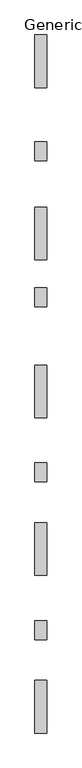
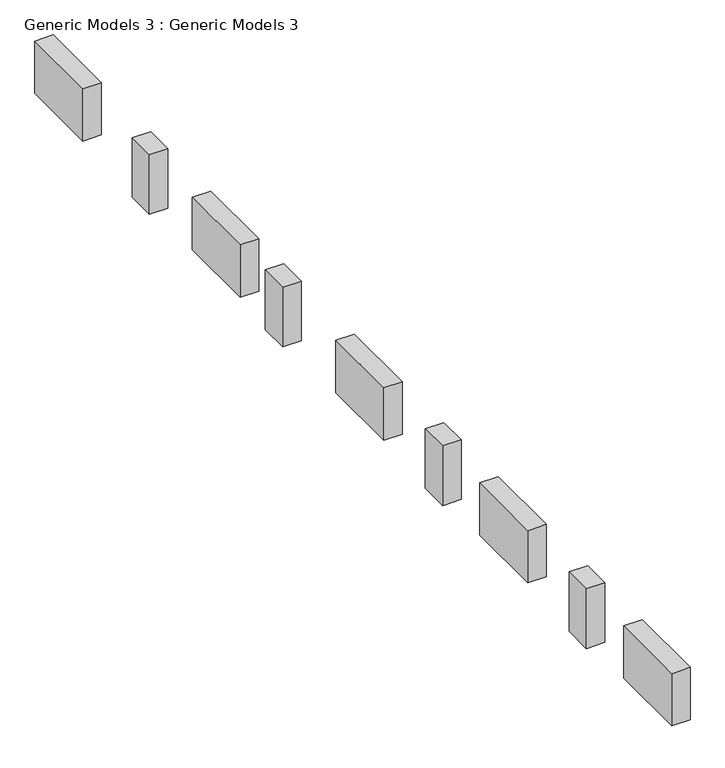
"""IFC4 building model written with IfcOpenShell, lengths in millimetres: proxy geometry, Generic Models 3 : Generic Models 3."""

from ifc_helpers import new_model, si_unit, frame, origin, place, context, project, spatial, polyline, outline, extrude, source, transform, mapped, element, save


def generic_models_3_generic_models_3_98a77e8e(model_context):
    return source(origin(), model_context, "Body", "SweptSolid", [
        extrude(outline(polyline([(5820.7206788, -7364.0778318), (5820.7206788, -8735.6778318), (5515.9206788, -8735.6778318), (5515.9206788, -7364.0778318), (5820.7206788, -7364.0778318)])), frame((0.0, 0.0, 262.9036405), z_axis=(0.0, 0.0, 1.0), x_axis=(1.0, 0.0, 0.0)), (0.0, 0.0, 1.0), 914.4),
        extrude(outline(polyline([(5820.7206788, -5805.4564015), (5820.7206788, -6300.7628124), (5515.9206788, -6300.7628124), (5515.9206788, -5805.4564015), (5820.7206788, -5805.4564015)])), frame((0.0, 0.0, 137.1997889), z_axis=(0.0, 0.0, 1.0), x_axis=(1.0, 0.0, 0.0)), (0.0, 0.0, 1.0), 1040.1038516),
        extrude(outline(polyline([(5820.7206788, -3249.2778318), (5820.7206788, -4620.8778318), (5515.9206788, -4620.8778318), (5515.9206788, -3249.2778318), (5820.7206788, -3249.2778318)])), frame((0.0, 0.0, 262.9036405), z_axis=(0.0, 0.0, 1.0), x_axis=(1.0, 0.0, 0.0)), (0.0, 0.0, 1.0), 914.4),
        extrude(outline(polyline([(5820.7206788, 862.0435985), (5820.7206788, -509.5564015), (5515.9206788, -509.5564015), (5515.9206788, 862.0435985), (5820.7206788, 862.0435985)])), frame((0.0, 0.0, 262.9036405), z_axis=(0.0, 0.0, 1.0), x_axis=(1.0, 0.0, 0.0)), (0.0, 0.0, 1.0), 914.4),
        extrude(outline(polyline([(5820.7206788, 4976.8435985), (5820.7206788, 3605.2435985), (5515.9206788, 3605.2435985), (5515.9206788, 4976.8435985), (5820.7206788, 4976.8435985)])), frame((0.0, 0.0, 262.9036405), z_axis=(0.0, 0.0, 1.0), x_axis=(1.0, 0.0, 0.0)), (0.0, 0.0, 1.0), 914.4),
        extrude(outline(polyline([(5820.7206788, 9472.6435985), (5820.7206788, 8101.0435985), (5515.9206788, 8101.0435985), (5515.9206788, 9472.6435985), (5820.7206788, 9472.6435985)])), frame((0.0, 0.0, 262.9036405), z_axis=(0.0, 0.0, 1.0), x_axis=(1.0, 0.0, 0.0)), (0.0, 0.0, 1.0), 914.4),
        extrude(outline(polyline([(5820.7206788, -1690.6564015), (5820.7206788, -2185.9628124), (5515.9206788, -2185.9628124), (5515.9206788, -1690.6564015), (5820.7206788, -1690.6564015)])), frame((0.0, 0.0, 137.1997889), z_axis=(0.0, 0.0, 1.0), x_axis=(1.0, 0.0, 0.0)), (0.0, 0.0, 1.0), 1040.1038516),
        extrude(outline(polyline([(5820.7206788, 2881.3435985), (5820.7206788, 2386.0371876), (5515.9206788, 2386.0371876), (5515.9206788, 2881.3435985), (5820.7206788, 2881.3435985)])), frame((0.0, 0.0, 137.1997889), z_axis=(0.0, 0.0, 1.0), x_axis=(1.0, 0.0, 0.0)), (0.0, 0.0, 1.0), 1040.1038516),
        extrude(outline(polyline([(5820.7206788, 6691.3435985), (5820.7206788, 6196.0371876), (5515.9206788, 6196.0371876), (5515.9206788, 6691.3435985), (5820.7206788, 6691.3435985)])), frame((0.0, 0.0, 137.1997889), z_axis=(0.0, 0.0, 1.0), x_axis=(1.0, 0.0, 0.0)), (0.0, 0.0, 1.0), 1040.1038516),
    ])


if __name__ == "__main__":
    model = new_model("IFC4")
    model_context = context("Model", 3, world=origin())
    ifc_project = project(units=[si_unit("LENGTHUNIT", "METRE", prefix="MILLI")], contexts=[model_context])
    site = spatial("IfcSite", under=ifc_project)
    building = spatial("IfcBuilding", under=site)
    placement = place(None, origin())
    generic_models_3_generic_models_3_shape = generic_models_3_generic_models_3_98a77e8e(model_context)
    element("IfcBuildingElementProxy", 1, Name="Generic Models 3 : Generic Models 3", ObjectType="Generic Models 3 : Generic Models 3", at=placement, inside=building, context=model_context, shape_type="MappedRepresentation", body=[
        mapped(generic_models_3_generic_models_3_shape, transform((0.0, 0.0, 0.0), x_axis=(1.0, 0.0, 0.0), y_axis=(0.0, 1.0, 0.0), z_axis=(0.0, 0.0, 1.0))),
    ])
    save(model, "model.ifc")

# Revit data of these elements
# Element 1 (IfcBuildingElementProxy, "Generic Models 3 : Generic Models 3")
#   Materials on its faces: "Parking Stripe"
# Materials
#   "Parking Stripe": class "Paint", colour RGB 250 250 91, transparency 0, Cost = 0
